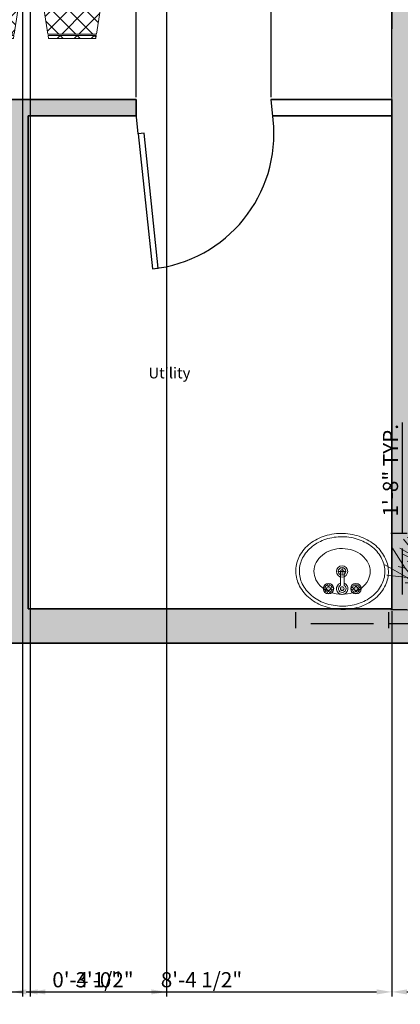
# Model space of a CAD drawing. Units: inches. Extents: x 1872 to 2380, y 714 to 1327.
# Tile 2 of 9: x 2100 to 2200, y 714 to 974. Entities that reach past the tile are written whole.
import ezdxf

# ---------------------------------------------------------------- set-up
doc = ezdxf.new("R2010")
doc.units = ezdxf.units.IN
doc.linetypes.add('HIDDEN', pattern=[9.525, 6.35, -3.175])
for name, color, linetype, lineweight in [('A-ANNO-DIMS', 2, 'Continuous', 18), ('A-AREA-IDEN', 7, 'Continuous', 18), ('A-DOOR', 4, 'Continuous', 25), ('A-FLOR-FIXT', 9, 'Continuous', 20), ('A-FURN', 8, 'Continuous', 18), ('A-WALL', 7, 'Continuous', 35), ('A-WALL-HIDN', 7, 'HIDDEN', 18), ('L-PLNT', 3, 'Continuous', 13)]:
    doc.layers.add(name, color=color, linetype=linetype, lineweight=lineweight)
for name, color, linetype, lineweight, true_color in [('A-FLOR-FIXT-PATT', 7, 'Continuous', 13, 0xd1ffff), ('A-FURN-PATT', 254, 'Continuous', 13, 0xf8ceb3), ('A-WALL-PATT', 242, 'Continuous', 13, 0xd52e31)]:
    doc.layers.add(name, color=color, linetype=linetype, lineweight=lineweight, true_color=true_color)
doc.styles.get("Standard").update_dxf_attribs({"font": 'arial.ttf'})
doc.dimstyles.new('ISO-25', dxfattribs={"dimtxt": 4, "dimasz": 4, "dimexe": 1.25, "dimexo": 0.625, "dimtad": 1, "dimdec": 0, "dimlunit": 3, "dimtxsty": 'Standard', "dimcen": 2.5, "dimadec": 0, "dimazin": 0, "dimtfac": 1, "dimtdec": 0, "dimtmove": 0, "dimatfit": 3, "dimfxl": 1, "dimarcsym": 0})

# ---------------------------------------------------------------- blocks, each defined once
blk = doc.blocks.new('*U5')
at = {"transparency": 33554687}
for p, q in [((0, 0), (0, -6)), ((-40, 0), (-40, -6))]:
    blk.add_line(p, q, dxfattribs=at)
blk.add_lwpolyline([(0, 0), (0, 40), (-1.75, 40), (-1.75, 0)], close=True, dxfattribs=at)
blk.add_arc((0, 0), 40, 90, 180, dxfattribs=at)
blk = doc.blocks.new('Sink - Oval top')
for p, q in [((-1, 0), (1, 0)), ((0, 1), (0, -1))]:
    blk.add_line(p, q)
for points in [[(-12.23, 0.39, 0.117634), (-11.46, -3.36, 0.104469), (-8.88, -6.8, 0.090016), (-5.08, -9.07, 0.08192), (-0.32, -10.02, 0.08192), (4.49, -9.38, 0.090016), (8.42, -7.36, 0.104469), (11.22, -4.09, 0.117634), (12.23, -0.39, 0.117634), (11.46, 3.36, 0.104469), (8.88, 6.8, 0.090016), (5.08, 9.07, 0.08192), (0.32, 10.02, 0.08192), (-4.49, 9.38, 0.090016), (-8.42, 7.36, 0.104469), (-11.22, 4.09, 0.117634)], [(-11.29, 0.16, 0.118622), (-10.52, -3.25, 0.104678), (-8.07, -6.36, 0.089562), (-4.54, -8.37, 0.081185), (-0.13, -9.15, 0.081185), (4.3, -8.49, 0.089562), (7.89, -6.58, 0.104678), (10.42, -3.55, 0.118622), (11.29, -0.16, 0.118622), (10.52, 3.25, 0.104678), (8.07, 6.36, 0.089562), (4.54, 8.37, 0.081185), (0.13, 9.15, 0.081185), (-4.3, 8.49, 0.089562), (-7.89, 6.58, 0.104678), (-10.42, 3.55, 0.118622)], [(-7.42, 0.08, 0.118283), (-6.91, -2.17, 0.104607), (-5.29, -4.21, 0.089718), (-2.97, -5.53, 0.081436), (-0.07, -6.04, 0.081436), (2.84, -5.59, 0.089718), (5.2, -4.33, 0.104607), (6.86, -2.32, 0.118283), (7.42, -0.08, 0.118283), (6.91, 2.17, 0.104607), (5.29, 4.21, 0.089718), (2.97, 5.53, 0.081436), (0.07, 6.04, 0.081436), (-2.84, 5.59, 0.089718), (-5.2, 4.33, 0.104607), (-6.86, 2.32, 0.118283)]]:
    blk.add_lwpolyline(points, format="xyb", close=True)
for radius in [1.5, 1]:
    blk.add_circle((0, 0), radius)
blk = doc.blocks.new('Dining Set - 36 x 72 in.')
for p, q in [((-22, 27.5), (-22.1562, 26.50042)), ((-22, 27.5), (-6, 27.5)), ((-5.8437, 26.49966), (-6, 27.5)), ((6, 27.5), (5.8438, 26.50042)), ((6, 27.5), (22, 27.5)), ((22.1563, 26.49966), (22, 27.5)), ((-22.2343, 26.00059), (-23.4847, 17.99762)), ((-22.2304, 26), (-5.7608, 26)), ((-5.8416, 26.5), (-22.1534, 26.5)), ((-4.5152, 17.99762), (-5.7655, 25.99926)), ((5.7657, 26.00059), (4.5153, 17.99762)), ((5.7696, 26), (22.2392, 26)), ((22.1584, 26.5), (5.8466, 26.5)), ((23.4848, 17.99762), (22.2345, 25.99926)), ((36, 18), (-36, 18)), ((-36, 18), (-36, -18)), ((36, -18), (36, 18)), ((-45.5, 8), (-44.5004, 8.15617)), ((-45.5, 8), (-45.5, -8)), ((-44.5, -8.15843), (-44.5, 8.15338)), ((-44.0006, 8.23428), (-35.9976, 9.48474)), ((-44, 8.23041), (-44, -8.23915)), ((44.0006, 8.23428), (35.9976, 9.48474)), ((44, 8.23041), (44, -8.23915)), ((44.5, -8.15843), (44.5, 8.15338)), ((45.5, 8), (44.5005, 8.15617)), ((45.5, 8), (45.5, -8)), ((-44.4997, -8.15631), (-45.5, -8)), ((-35.9976, -9.48476), (-43.9993, -8.2345)), ((35.9976, -9.48476), (43.9993, -8.2345)), ((44.4997, -8.15631), (45.5, -8)), ((-36, -18), (36, -18)), ((-22.2343, -26.0006), (-23.4847, -17.99762)), ((-4.5152, -17.99762), (-5.7655, -25.99928)), ((5.7657, -26.0006), (4.5153, -17.99762)), ((23.4848, -17.99762), (22.2345, -25.99928)), ((-22.2304, -26), (-5.7608, -26)), ((-22, -27.5), (-22.1562, -26.50044)), ((-5.8416, -26.5), (-22.1534, -26.5)), ((-5.8437, -26.49967), (-6, -27.5)), ((5.7696, -26), (22.2392, -26)), ((6, -27.5), (5.8438, -26.50044)), ((22.1584, -26.5), (5.8466, -26.5)), ((22.1563, -26.49967), (22, -27.5)), ((-22, -27.5), (-6, -27.5)), ((6, -27.5), (22, -27.5))]:
    blk.add_line(p, q)
for points in [[(-36, 15), (-31.1772, 14.97754), (-26.8079, 14.91406), (-22.8538, 14.81543), (-19.276, 14.6875), (-16.0362, 14.53613), (-13.0957, 14.36718), (-10.4159, 14.18652), (-7.9583, 14), (-5.6904, 13.81315), (-3.6035, 13.63021), (-1.6954, 13.45508), (0.0365, 13.29166), (1.5945, 13.14388), (2.9811, 13.01562), (4.1988, 12.9108), (5.25, 12.83333), (6.1393, 12.78613), (6.8802, 12.76823), (7.4883, 12.77767), (7.9792, 12.8125), (8.3685, 12.87077), (8.6719, 12.95052), (8.9049, 13.0498), (9.0833, 13.16666), (9.2205, 13.29899), (9.3216, 13.44401), (9.3895, 13.59879), (9.4271, 13.76041), (9.4373, 13.92594), (9.4232, 14.09245), (9.3875, 14.257), (9.3333, 14.41666), (9.2638, 14.56917), (9.1836, 14.71484), (9.0975, 14.85465), (9.0104, 14.98958), (8.9272, 15.1206), (8.8529, 15.2487), (8.7922, 15.37483), (8.75, 15.5), (8.7305, 15.62467), (8.7344, 15.74739), (8.7617, 15.86621), (8.8125, 15.97916), (8.8867, 16.08431), (8.9844, 16.17968), (9.1055, 16.26334), (9.25, 16.33333), (9.4189, 16.38802), (9.6172, 16.42708), (9.8506, 16.45052), (10.125, 16.45833), (10.4463, 16.45052), (10.8203, 16.42708), (11.2529, 16.38802), (11.75, 16.33333), (12.3184, 16.26318), (12.9694, 16.17838), (13.7151, 16.07991), (14.5677, 15.96875), (15.5395, 15.84586), (16.6426, 15.71224), (17.8893, 15.56884), (19.2917, 15.41666), (20.859, 15.25667), (22.5879, 15.08984), (24.4721, 14.91715), (26.5052, 14.73958), (28.6809, 14.5581), (30.9929, 14.3737), (33.4347, 14.18733), (36, 14)], [(-36, 10), (-28.9766, 10.14274), (-23.1725, 10.20442), (-18.4241, 10.19775), (-14.5677, 10.13541), (-11.4399, 10.03011), (-8.877, 9.89453), (-6.7154, 9.74137), (-4.7917, 9.58333), (-2.9698, 9.43082), (-1.2246, 9.28515), (0.4415, 9.14534), (2.026, 9.01041), (3.5266, 8.87939), (4.9408, 8.7513), (6.266, 8.62516), (7.5, 8.5), (8.6411, 8.37549), (9.6914, 8.2539), (10.6538, 8.13818), (11.5312, 8.03125), (12.3267, 7.93603), (13.043, 7.85547), (13.6831, 7.79248), (14.25, 7.75), (14.7471, 7.7303), (15.1797, 7.73307), (15.5537, 7.75732), (15.875, 7.80208), (16.1494, 7.86637), (16.3828, 7.94922), (16.5811, 8.04964), (16.75, 8.16666), (16.8944, 8.29915), (17.0143, 8.44531), (17.1089, 8.60319), (17.1771, 8.77083), (17.218, 8.94629), (17.2305, 9.1276), (17.2137, 9.31282), (17.1667, 9.5), (17.0895, 9.6875), (16.987, 9.875), (16.8649, 10.0625), (16.7292, 10.25), (16.5856, 10.4375), (16.4401, 10.625), (16.2985, 10.8125), (16.1667, 11), (16.05, 11.18733), (15.9518, 11.3737), (15.8752, 11.5581), (15.8229, 11.73958), (15.798, 11.91715), (15.8034, 12.08984), (15.842, 12.25667), (15.9167, 12.41666), (16.0295, 12.56836), (16.1784, 12.70833), (16.3605, 12.83268), (16.5729, 12.9375), (16.8127, 13.01888), (17.0768, 13.07291), (17.3625, 13.0957), (17.6667, 13.08333), (17.9894, 13.03312), (18.3418, 12.94726), (18.7382, 12.82918), (19.1927, 12.68229), (19.7195, 12.51001), (20.3327, 12.31575), (21.0465, 12.10294), (21.875, 11.875), (22.8357, 11.63354), (23.959, 11.37304), (25.2786, 11.08618), (26.8282, 10.76562), (28.6414, 10.40405), (30.752, 9.99414), (33.1936, 9.52856), (36, 9)], [(-36, 5.5), (-30.7157, 5.3348), (-26.069, 5.20963), (-21.9946, 5.11767), (-18.4271, 5.05208), (-15.3009, 5.00602), (-12.5508, 4.97265), (-10.1112, 4.94515), (-7.9167, 4.91666), (-5.909, 4.88167), (-4.0586, 4.83984), (-2.3429, 4.79215), (-0.7396, 4.73958), (0.7739, 4.6831), (2.22, 4.6237), (3.6213, 4.56233), (5, 4.5), (6.373, 4.43782), (7.7344, 4.3776), (9.0723, 4.32129), (10.375, 4.27083), (11.6309, 4.22819), (12.8281, 4.19531), (13.9551, 4.17415), (15, 4.16666), (15.954, 4.17448), (16.819, 4.19791), (17.6001, 4.23698), (18.3021, 4.29166), (18.9299, 4.36198), (19.4883, 4.44791), (19.9823, 4.54948), (20.4167, 4.66666), (20.7969, 4.79899), (21.1302, 4.94401), (21.4245, 5.09879), (21.6875, 5.26041), (21.9271, 5.42594), (22.1511, 5.59245), (22.3672, 5.757), (22.5834, 5.91666), (22.8065, 6.06868), (23.0404, 6.21093), (23.2879, 6.34147), (23.5521, 6.45833), (23.8358, 6.55957), (24.142, 6.64323), (24.4735, 6.70735), (24.8334, 6.75), (25.2235, 6.76969), (25.642, 6.76692), (26.0858, 6.74267), (26.5521, 6.69791), (27.0379, 6.63362), (27.5404, 6.55078), (28.0565, 6.45036), (28.5834, 6.33333), (29.1242, 6.19987), (29.7071, 6.04687), (30.3661, 5.87044), (31.1354, 5.66666), (32.0493, 5.43164), (33.142, 5.16146), (34.4475, 4.85221), (36, 4.5)], [(-36, -1), (-30.7915, -0.6591), (-26.0195, -0.38216), (-21.6519, -0.16284), (-17.6563, 0.00521), (-14.0005, 0.12833), (-10.6523, 0.21289), (-7.5796, 0.26522), (-4.75, 0.29166), (-2.134, 0.29793), (0.2878, 0.28711), (2.5317, 0.26163), (4.6146, 0.22396), (6.5529, 0.17651), (8.3633, 0.12174), (10.0623, 0.06209), (11.6667, 0), (13.1899, -0.06201), (14.6341, -0.1211), (15.9982, -0.17432), (17.2813, -0.21875), (18.4823, -0.25147), (19.6003, -0.26953), (20.6343, -0.27002), (21.5834, -0.25), (22.4481, -0.20768), (23.2357, -0.14584), (23.9549, -0.06836), (24.6146, 0.02083), (25.2235, 0.11784), (25.7904, 0.21875), (26.3241, 0.31966), (26.8334, 0.41666), (27.3265, 0.50618), (27.8099, 0.58593), (28.2894, 0.65397), (28.7709, 0.70833), (29.2601, 0.74707), (29.763, 0.76823), (30.2855, 0.76985), (30.8334, 0.75), (31.4088, 0.70784), (31.9994, 0.64713), (32.589, 0.57275), (33.1615, 0.48958), (33.7008, 0.4025), (34.1908, 0.3164), (34.6153, 0.23616), (34.9584, 0.16666), (35.2099, 0.11165), (35.3848, 0.07031), (35.504, 0.04069), (35.5886, 0.02083), (35.6594, 0.00879), (35.7377, 0.0026), (35.8442, 0.00032), (36, 0)], [(-36, -6.5), (-27.1843, -6.31267), (-20.084, -6.1263), (-14.469, -5.9419), (-10.1094, -5.76042), (-6.7752, -5.58285), (-4.2363, -5.41016), (-2.2629, -5.24333), (-0.625, -5.08334), (0.8708, -4.93099), (2.2715, -4.78646), (3.5872, -4.64974), (4.8281, -4.52084), (6.0046, -4.39974), (7.127, -4.28646), (8.2053, -4.18099), (9.25, -4.08334), (10.2705, -3.99382), (11.2734, -3.91407), (12.2647, -3.84603), (13.25, -3.79167), (14.2354, -3.75293), (15.2266, -3.73177), (16.2295, -3.73015), (17.25, -3.75), (18.2912, -3.79248), (19.3451, -3.85547), (20.4009, -3.93604), (21.4479, -4.03125), (22.4754, -4.13819), (23.4727, -4.25391), (24.4289, -4.37549), (25.3334, -4.5), (26.1785, -4.62492), (26.9694, -4.74935), (27.7145, -4.87281), (28.4219, -4.99479), (29.1, -5.11483), (29.7572, -5.23242), (30.4016, -5.34709), (31.0417, -5.45834), (31.6837, -5.56437), (32.3262, -5.65821), (32.9658, -5.73153), (33.599, -5.77604), (34.2224, -5.78345), (34.8327, -5.74545), (35.4264, -5.65373), (36, -5.5)], [(-36, -10), (-26.4022, -9.81299), (-18.4675, -9.62891), (-11.9839, -9.45069), (-6.7396, -9.28125), (-2.5226, -9.12354), (0.8789, -8.98047), (3.6769, -8.85498), (6.0833, -8.75), (8.2767, -8.66765), (10.3021, -8.60677), (12.1712, -8.56543), (13.8958, -8.54167), (15.4876, -8.53353), (16.9583, -8.53907), (18.3197, -8.55632), (19.5834, -8.58334), (20.7616, -8.61841), (21.8685, -8.66081), (22.9188, -8.71004), (23.9271, -8.76563), (24.9081, -8.82707), (25.8763, -8.89388), (26.8465, -8.96558), (27.8334, -9.04167), (28.8474, -9.12118), (29.8828, -9.20117), (30.93, -9.27824), (31.9792, -9.34896), (33.0205, -9.40991), (34.0443, -9.45768), (35.0407, -9.48885), (36, -9.5)], [(-36, -14.5), (-30.0881, -14.33513), (-25.0332, -14.21224), (-20.7312, -14.12647), (-17.0781, -14.07292), (-13.97, -14.04671), (-11.3027, -14.04297), (-8.9724, -14.05681), (-6.875, -14.08334), (-4.9224, -14.11833), (-3.0905, -14.16016), (-1.3709, -14.20785), (0.2448, -14.26042), (1.7647, -14.3169), (3.1973, -14.3763), (4.5507, -14.43767), (5.8333, -14.5), (7.0554, -14.5621), (8.235, -14.62175), (9.3922, -14.67652), (10.5469, -14.72396), (11.7192, -14.76164), (12.929, -14.78711), (14.1965, -14.79794), (15.5417, -14.79167), (16.9933, -14.76424), (18.6152, -14.70508), (20.4804, -14.60197), (22.6615, -14.44271), (25.2312, -14.21509), (28.2624, -13.9069), (31.8277, -13.50594), (36, -13)]]:
    blk.add_lwpolyline(points)
blk = doc.blocks.new('Faucet - Bathroom top')
for p, q in [((-4.107, 0.125), (-4.375, 0.125)), ((-3.75, 0.4788), (-3.75, 0.75)), ((-3.5, 0.482), (-3.5, 0.75)), ((-3.1461, 0.125), (-2.875, 0.125)), ((3.143, 0.125), (2.875, 0.125)), ((3.5, 0.4788), (3.5, 0.75)), ((3.75, 0.482), (3.75, 0.75)), ((4.1039, 0.125), (4.375, 0.125)), ((-4.1039, -0.125), (-4.375, -0.125)), ((-3.75, -0.4821), (-3.75, -0.75)), ((-3.5, -0.4789), (-3.5, -0.75)), ((-3.143, -0.125), (-2.875, -0.125)), ((-0.5, -0.8639), (-0.5, -4.5)), ((0.5, -4.5), (0.5, -0.8631)), ((3.1461, -0.125), (2.875, -0.125)), ((3.5, -0.4821), (3.5, -0.75)), ((3.75, -0.4789), (3.75, -0.75)), ((4.107, -0.125), (4.375, -0.125))]:
    blk.add_line(p, q)
for centre, radius in [((-3.625, 0), 1.375), ((-4.625, 0), 0.2795), ((-3.625, 0), 0.5), ((-3.625, 1), 0.2795), ((-2.625, 0), 0.2795), ((0, 0), 0.5), ((3.625, 0), 1.375), ((2.625, 0), 0.2795), ((3.625, 0), 0.5), ((3.625, 1), 0.2795), ((4.625, 0), 0.2795), ((-3.625, -1), 0.2795), ((3.625, -1), 0.2795)]:
    blk.add_circle(centre, radius)
for centre, radius, start, end in [((-3.625, 0), 1, 105.2407, 164.2093), ((-3.625, 0), 1, 16.44125, 74.07887), ((0, 0), 1.5, 289.6514, 250.3603), ((0, 0), 1, 300.3431, 239.7554), ((3.625, 0), 1, 106.12, 164.0884), ((3.625, 0), 1, 16.23422, 73.90469), ((-3.625, 0), 1, 196.2342, 253.9047), ((-3.625, 0), 1, 286.12, 344.0884), ((3.625, 0), 1, 196.4413, 254.0789), ((3.625, 0), 1, 285.2407, 344.2093), ((0, -4.5), 0.5, 180, 0)]:
    blk.add_arc(centre, radius, start, end)
blk = doc.blocks.new('*U18')
for p, q in [((-316.7634, 502.285), (-327.6092, 559.9176)), ((-286.512, 498.3226), (-307.4416, 538.0736)), ((-290.3982, 464.5406), (-265.6078, 577.8246)), ((-207.264, 451.104), (-268.224, 548.64)), ((-240.792, 502.285), (-228.3968, 573.8368)), ((-182.88, 499.872), (-158.496, 536.448)), ((-129.1844, 450.6214), (-140.0302, 542.036)), ((-134.112, 487.68), (-97.536, 548.64)), ((-85.7758, 472.4908), (-73.3552, 548.005)), ((-12.9032, 555.9552), (-2.0574, 522.1732)), ((-5.1562, 486.3846), (2.5908, 542.036)), ((-0.508, 508.254), (22.7584, 536.067)), ((1.0414, 526.1356), (35.1536, 559.9176)), ((2.5908, 542.036), (21.209, 555.9552)), ((-426.72, 414.528), (-475.488, 475.488)), ((-377.952, 463.296), (-451.104, 487.68)), ((-426.72, 414.528), (-390.144, 499.872)), ((-377.952, 463.296), (-329.184, 524.256)), ((-207.264, 304.8), (-377.952, 463.296)), ((-338.455, 424.7896), (-290.3982, 464.5406)), ((-296.5958, 484.4034), (-316.7634, 502.285)), ((-305.8922, 396.9512), (-302.7934, 478.4344)), ((-302.7934, 478.4344), (-270.256, 518.1854)), ((-268.7066, 458.5716), (-250.0884, 500.3038)), ((-182.88, 499.872), (-219.456, 512.064)), ((-207.264, 451.104), (-134.112, 487.68)), ((-121.92, 414.528), (-182.88, 499.872)), ((-73.152, 329.184), (-109.728, 499.872)), ((-97.536, 426.72), (-24.384, 524.256)), ((-70.2564, 426.7708), (-85.7758, 472.4908)), ((-73.152, 402.336), (-60.96, 512.064)), ((8.7884, 335.3562), (-5.1562, 486.3846)), ((-3.6068, 492.3536), (14.986, 518.1854)), ((33.6042, 412.8516), (92.5068, 464.5406)), ((-463.296, 280.416), (-552.577, 423.037)), ((-329.184, 316.992), (-499.872, 414.528)), ((-426.72, 316.992), (-426.72, 414.528)), ((-329.184, 316.992), (-207.264, 451.104)), ((-304.3428, 426.7708), (-268.7066, 458.5716)), ((-182.88, 377.952), (-97.536, 426.72)), ((-85.7758, 389.001), (-129.1844, 452.6026)), ((-24.384, 268.224), (-73.152, 402.336)), ((8.7884, 335.3562), (33.6042, 412.8516)), ((36.576, 390.144), (73.152, 438.912)), ((60.96, 390.144), (85.344, 414.528)), ((-353.568, 316.992), (-487.68, 377.952)), ((-195.072, 316.992), (-182.88, 377.952)), ((-12.192, 274.32), (8.7884, 335.3562)), ((24.384, 304.8), (36.576, 390.144)), ((24.384, 304.8), (73.152, 377.952)), ((48.768, 341.376), (60.96, 390.144)), ((-451.104, 219.456), (-601.0402, 303.8094)), ((-463.296, 280.416), (-512.064, 292.608)), ((-402.336, 207.264), (-463.296, 280.416)), ((-426.72, 316.992), (-451.104, 329.184)), ((-402.336, 207.264), (-426.72, 316.992)), ((-329.184, 316.992), (-353.568, 316.992)), ((-268.224, 109.728), (-329.184, 316.992)), ((-219.456, 195.072), (-207.264, 304.8)), ((-170.688, 219.456), (-195.072, 316.992)), ((-85.344, 134.112), (-73.152, 329.184)), ((-48.768, 243.84), (24.384, 304.8)), ((-451.104, 219.456), (-587.4512, 234.2388)), ((-377.952, 146.304), (-451.104, 219.456)), ((-377.952, 146.304), (-402.336, 207.264)), ((-146.304, 134.112), (-170.688, 219.456)), ((-109.728, 73.152), (-48.768, 243.84)), ((-414.528, 182.88), (-463.296, 182.88)), ((-329.184, 121.92), (-377.952, 146.304)), ((-268.224, 109.728), (-219.456, 195.072)), ((-158.496, 73.152), (-146.304, 134.112)), ((-292.608, 60.96), (-329.184, 121.92)), ((-219.456, 48.768), (-268.224, 109.728)), ((-219.456, 24.384), (-109.728, 73.152)), ((-219.456, 24.384), (-158.496, 73.152)), ((-402.336, 12.192), (-451.104, 0)), ((-341.376, 12.192), (-402.336, 12.192)), ((-243.84, 24.384), (-341.376, 12.192)), ((-243.84, 24.384), (-329.184, 0)), ((-219.456, 24.384), (-292.608, 60.96)), ((-243.84, 24.384), (-195.072, 24.384)), ((-219.456, 24.384), (-219.456, 48.768)), ((-219.456, 24.384), (-73.152, 24.384)), ((-195.072, 24.384), (-158.496, 12.192)), ((-158.496, 12.192), (-85.344, 0)), ((-73.152, 24.384), (0, 0))]:
    blk.add_line(p, q)
blk = doc.blocks.new('*D30')
at = {"layer": 'A-ANNO-DIMS', "color": 0, "lineweight": -2, "transparency": 16777216}
for p, q in [((2172.51, 817.84), (2172.51, 813.54)), ((2197.06, 817.84), (2197.06, 813.54)), ((2176.51, 814.79), (2193.06, 814.79)), ((2197.06, 814.79), (2254.16, 814.79))]:
    blk.add_line(p, q, dxfattribs=at)
at = {"layer": 'A-ANNO-DIMS', "color": 0, "transparency": 16777216}
for points in [[(2176.51, 815.45), (2176.51, 814.12), (2172.51, 814.79)], [(2193.06, 815.45), (2193.06, 814.12), (2197.06, 814.79)]]:
    blk.add_solid(points, dxfattribs=at)
at = {"layer": 'Defpoints', "color": 0, "transparency": 16777216}
for p in [(2172.51, 818.47), (2197.06, 818.47), (2197.06, 814.79)]:
    blk.add_point(p, dxfattribs=at)
at = {"layer": 'A-ANNO-DIMS', "color": 0, "transparency": 16777216, "insert": (2227.61, 817.48), "char_height": 4, "attachment_point": 5}
blk.add_mtext('BASIN 2\'-0 1/2" TYP.', dxfattribs=at)
blk = doc.blocks.new('*D31')
at = {"layer": 'A-ANNO-DIMS', "color": 0, "lineweight": -2, "transparency": 16777216}
for p, q in [((2200.74, 838.61), (2200.74, 867.86)), ((2197.68, 838.61), (2201.99, 838.61)), ((2200.74, 822.47), (2200.74, 834.61)), ((2197.68, 818.47), (2201.99, 818.47))]:
    blk.add_line(p, q, dxfattribs=at)
at = {"layer": 'A-ANNO-DIMS', "color": 0, "transparency": 16777216}
for points in [[(2200.07, 834.61), (2201.41, 834.61), (2200.74, 838.61)], [(2200.07, 822.47), (2201.41, 822.47), (2200.74, 818.47)]]:
    blk.add_solid(points, dxfattribs=at)
at = {"layer": 'Defpoints', "color": 0, "transparency": 16777216}
for p in [(2197.06, 838.61), (2200.74, 838.61), (2197.06, 818.47)]:
    blk.add_point(p, dxfattribs=at)
at = {"layer": 'A-ANNO-DIMS', "color": 0, "transparency": 16777216, "insert": (2198.07, 855.23), "char_height": 4, "attachment_point": 5, "rotation": 90}
blk.add_mtext('1\'-8" TYP.', dxfattribs=at)
blk = doc.blocks.new('*D60')
at = {"layer": 'A-ANNO-DIMS', "color": 0, "lineweight": -2, "transparency": 16777216}
for p, q in [((2097.4, 818.02), (2097.4, 716.39)), ((2197.9, 818.02), (2197.9, 716.39)), ((2101.4, 717.64), (2193.9, 717.64))]:
    blk.add_line(p, q, dxfattribs=at)
at = {"layer": 'A-ANNO-DIMS', "color": 0, "transparency": 16777216}
for points in [[(2101.4, 718.3), (2101.4, 716.97), (2097.4, 717.64)], [(2193.9, 718.3), (2193.9, 716.97), (2197.9, 717.64)]]:
    blk.add_solid(points, dxfattribs=at)
at = {"layer": 'Defpoints', "color": 0, "transparency": 16777216}
for p in [(2097.4, 818.64), (2197.9, 818.64), (2197.9, 717.64)]:
    blk.add_point(p, dxfattribs=at)
at = {"layer": 'A-ANNO-DIMS', "color": 0, "transparency": 16777216, "insert": (2147.65, 720.33), "char_height": 4, "attachment_point": 5}
blk.add_mtext('8\'-4 1/2"', dxfattribs=at)
blk = doc.blocks.new('*D61')
at = {"layer": 'A-ANNO-DIMS', "color": 0, "lineweight": -2, "transparency": 16777216}
for p, q in [((2197.9, 818.02), (2197.9, 716.39)), ((2295.4, 809.02), (2295.4, 716.39)), ((2201.9, 717.64), (2291.4, 717.64))]:
    blk.add_line(p, q, dxfattribs=at)
at = {"layer": 'A-ANNO-DIMS', "color": 0, "transparency": 16777216}
for points in [[(2201.9, 718.3), (2201.9, 716.97), (2197.9, 717.64)], [(2291.4, 718.3), (2291.4, 716.97), (2295.4, 717.64)]]:
    blk.add_solid(points, dxfattribs=at)
at = {"layer": 'Defpoints', "color": 0, "transparency": 16777216}
for p in [(2197.9, 818.64), (2295.4, 809.64), (2295.4, 717.64)]:
    blk.add_point(p, dxfattribs=at)
at = {"layer": 'A-ANNO-DIMS', "color": 0, "transparency": 16777216, "insert": (2246.65, 720.33), "char_height": 4, "attachment_point": 5}
blk.add_mtext('8\'-1 1/2"', dxfattribs=at)
blk = doc.blocks.new('*D70')
at = {"layer": 'A-ANNO-DIMS', "color": 0, "lineweight": -2, "transparency": 16777216}
for p, q in [((2102.4, 1143.52), (2102.4, 716.39)), ((2138.4, 1143.52), (2138.4, 716.39)), ((2106.4, 717.64), (2134.4, 717.64))]:
    blk.add_line(p, q, dxfattribs=at)
at = {"layer": 'A-ANNO-DIMS', "color": 0, "transparency": 16777216}
for points in [[(2106.4, 718.3), (2106.4, 716.97), (2102.4, 717.64)], [(2134.4, 718.3), (2134.4, 716.97), (2138.4, 717.64)]]:
    blk.add_solid(points, dxfattribs=at)
at = {"layer": 'Defpoints', "color": 0, "transparency": 16777216}
for p in [(2102.4, 1144.14), (2138.4, 1144.14), (2138.4, 717.64)]:
    blk.add_point(p, dxfattribs=at)
at = {"layer": 'A-ANNO-DIMS', "color": 0, "transparency": 16777216, "insert": (2120.4, 720.31), "char_height": 4, "attachment_point": 5}
blk.add_mtext('3\'-0"', dxfattribs=at)
blk = doc.blocks.new('*D74')
at = {"layer": 'A-ANNO-DIMS', "color": 0, "lineweight": -2, "transparency": 16777216}
for p, q in [((2130.4, 953.62), (2130.4, 1319.69)), ((2166.01, 953.64), (2166.01, 1319.69)), ((2134.4, 1318.44), (2162.01, 1318.44))]:
    blk.add_line(p, q, dxfattribs=at)
at = {"layer": 'A-ANNO-DIMS', "color": 0, "transparency": 16777216}
for points in [[(2134.4, 1319.11), (2134.4, 1317.78), (2130.4, 1318.44)], [(2162.01, 1319.11), (2162.01, 1317.78), (2166.01, 1318.44)]]:
    blk.add_solid(points, dxfattribs=at)
at = {"layer": 'Defpoints', "color": 0, "transparency": 16777216}
for p in [(2166.01, 1318.44), (2130.4, 952.99), (2166.01, 953.01)]:
    blk.add_point(p, dxfattribs=at)
at = {"layer": 'A-ANNO-DIMS', "color": 0, "transparency": 16777216, "insert": (2148.2, 1321.14), "char_height": 4, "attachment_point": 5}
blk.add_mtext('2\'-11 1/2"', dxfattribs=at)
blk = doc.blocks.new('*D75')
at = {"layer": 'A-ANNO-DIMS', "color": 0, "lineweight": -2, "transparency": 16777216}
for p, q in [((2166.01, 953.64), (2166.02, 983.06)), ((2170.02, 981.81), (2193.91, 981.8)), ((2197.9, 953.62), (2197.91, 983.04))]:
    blk.add_line(p, q, dxfattribs=at)
at = {"layer": 'A-ANNO-DIMS', "color": 0, "transparency": 16777216}
for points in [[(2170.02, 982.48), (2170.02, 981.14), (2166.02, 981.81)], [(2193.91, 982.46), (2193.91, 981.13), (2197.91, 981.79)]]:
    blk.add_solid(points, dxfattribs=at)
at = {"layer": 'Defpoints', "color": 0, "transparency": 16777216}
for p in [(2197.91, 981.79), (2166.01, 953.01), (2197.9, 952.99)]:
    blk.add_point(p, dxfattribs=at)
at = {"layer": 'A-ANNO-DIMS', "color": 0, "transparency": 16777216, "insert": (2181.97, 984.47), "char_height": 4, "attachment_point": 5, "rotation": 359.9714}
blk.add_mtext('2\'-8"', dxfattribs=at)
blk = doc.blocks.new('*D80')
at = {"layer": 'A-ANNO-DIMS', "color": 0, "lineweight": -2, "transparency": 16777216}
for p, q in [((2095.9, 1112.15), (2095.9, 716.39)), ((2100.4, 1112.15), (2100.4, 716.39)), ((2091.9, 717.64), (2087.9, 717.64)), ((2095.9, 717.64), (2100.4, 717.64)), ((2104.4, 717.64), (2129.6, 717.64))]:
    blk.add_line(p, q, dxfattribs=at)
at = {"layer": 'A-ANNO-DIMS', "color": 0, "transparency": 16777216}
for points in [[(2091.9, 718.3), (2091.9, 716.97), (2095.9, 717.64)], [(2104.4, 718.3), (2104.4, 716.97), (2100.4, 717.64)]]:
    blk.add_solid(points, dxfattribs=at)
at = {"layer": 'Defpoints', "color": 0, "transparency": 16777216}
for p in [(2095.9, 1112.77), (2100.4, 1112.77), (2100.4, 717.64)]:
    blk.add_point(p, dxfattribs=at)
at = {"layer": 'A-ANNO-DIMS', "color": 0, "transparency": 16777216, "insert": (2119, 720.33), "char_height": 4, "attachment_point": 5}
blk.add_mtext('0\'-4 1/2"', dxfattribs=at)

msp = doc.modelspace()

# ---------------------------------------------------------------- hatches: boundary and pattern name
at = {"layer": 'A-FLOR-FIXT-PATT', "transparency": 33554687}
h = msp.add_hatch(color=256, dxfattribs=at)
h.dxf.hatch_style = 1
h.paths.add_polyline_path([(2155.91, 1229.14, 0.48008), (2138.39, 1226.79, 0.215004), (2138.39, 1223.5, 0.48008), (2155.91, 1221.14)])
h.paths.add_polyline_path([(2168.91, 1233.64, 0.5), (2167.91, 1234.64), (2163.91, 1234.64, 0.5), (2162.91, 1233.64), (2162.91, 1216.64, 0.5), (2163.91, 1215.64), (2167.91, 1215.64, 0.5), (2168.91, 1216.64)])
h.paths.add_polyline_path([(2285.4, 982.14, 0.5), (2284.4, 983.14), (2267.4, 983.14, 0.5), (2266.4, 982.14), (2266.4, 978.14, 0.5), (2267.4, 977.14), (2284.4, 977.14, 0.5), (2285.4, 978.14)])
h.paths.add_polyline_path([(2277.54, 1007.66, 0.215004), (2274.25, 1007.66, 0.48008), (2271.9, 990.14), (2279.9, 990.14, 0.48008)])
h.paths.add_polyline_path([(2285.9, 985.64), (2282.9, 985.64), (2282.9, 984.14), (2283.9, 984.14), (2283.9, 984.64), (2285.9, 984.64)])
h.paths.add_polyline_path([(2279.53, 1049.02, -0.039819), (2280.2, 1048.28, 0.216904), (2280.37, 1048.66, 0.658258)])
h.paths.add_polyline_path([(2279.53, 1049.02, 0.206085), (2279.37, 1048.66, 0.643515), (2280.2, 1048.28, 0.039819)])
h.paths.add_polyline_path([(2279.37, 1045.03, 1), (2280.37, 1045.03, 1)])
h.paths.add_polyline_path([(2280.37, 1041.41, 0.219955), (2280.19, 1041.79, -0.039801), (2279.52, 1041.05, 0.66578)])
h.paths.add_polyline_path([(2280.19, 1041.79, 0.639405), (2279.37, 1041.41, 0.200639), (2279.52, 1041.05, 0.039801)])
h.paths.add_polyline_path([(2158.34, 1154.61, 1), (2157.34, 1154.61, 1)])
h.paths.add_polyline_path([(2154.72, 1154.61, 1), (2153.72, 1154.61, 1)])
h.paths.add_polyline_path([(2161.97, 1154.61, 1), (2160.97, 1154.61, 1)])
h.paths.add_polyline_path([(2180.69, 824, 1), (2181.69, 824, 1)])
h.paths.add_polyline_path([(2185.32, 824, 1), (2184.32, 824, 1)])
h.paths.add_polyline_path([(2188.94, 824, 1), (2187.94, 824, 1)])
at = {"layer": 'A-FURN-PATT', "transparency": 33554687}
h = msp.add_hatch(dxfattribs=at)
h.set_pattern_fill('ANSI37', color=256)
h.paths.add_polyline_path([(2030.37, 1262.04), (1979.97, 1262.04), (1979.97, 1246.84), (1967.17, 1246.84), (1967.17, 1202.04), (2030.37, 1202.04)])
h.paths.add_polyline_path([(1964.77, 1246.84), (1966.77, 1248.84), (1966.77, 1254.04), (1951.57, 1254.04), (1951.57, 1233.24), (1964.77, 1233.24)])
h.paths.add_polyline_path([(1964.77, 1230.84), (1951.57, 1230.84), (1951.57, 1210.04), (1964.77, 1210.04)])
h.paths.add_polyline_path([(2268.08, 1263.68), (2221.12, 1263.68), (2221.12, 1219.09), (2258.57, 1219.09), (2258.57, 1230.39), (2268.08, 1230.39)])
h.paths.add_polyline_path([(2279.67, 1257.73), (2269.86, 1257.73), (2269.86, 1242.28), (2279.67, 1242.28)])
h.paths.add_polyline_path([(2279.67, 1240.49), (2269.86, 1240.49), (2269.86, 1230.39), (2268.38, 1228.9), (2268.38, 1225.04), (2279.67, 1225.04)])
h.paths.add_polyline_path([(2097.97, 1011.83), (2085.54, 1011.83), (2085.42, 1011.06), (2098.09, 1011.06)])
h.paths.add_polyline_path([(2098.15, 1010.67), (2085.36, 1010.67), (2084.39, 1004.45), (2099.13, 1004.45)])
h.paths.add_polyline_path([(2119.91, 1010.67), (2107.12, 1010.67), (2106.14, 1004.45), (2120.89, 1004.45)])
h.paths.add_polyline_path([(2119.73, 1011.83), (2107.3, 1011.83), (2107.18, 1011.06), (2119.85, 1011.06)])
h.paths.add_polyline_path([(2074.66, 997.83), (2068.44, 996.86), (2068.44, 984.06), (2074.66, 983.09)])
h.paths.add_polyline_path([(2068.05, 996.8), (2067.28, 996.68), (2067.28, 984.25), (2068.05, 984.12)])
h.paths.add_polyline_path([(2136.83, 996.86), (2130.61, 997.83), (2130.61, 983.09), (2136.83, 984.06)])
h.paths.add_polyline_path([(2137.99, 996.68), (2137.22, 996.8), (2137.22, 984.12), (2137.99, 984.25)])
h.paths.add_polyline_path([(2099.13, 976.47), (2084.39, 976.47), (2085.36, 970.26), (2098.15, 970.26)])
h.paths.add_polyline_path([(2120.89, 976.47), (2106.14, 976.47), (2107.12, 970.26), (2119.91, 970.26)])
h.paths.add_polyline_path([(2119.85, 969.87), (2107.18, 969.87), (2107.3, 969.09), (2119.73, 969.09)])
h.paths.add_polyline_path([(2098.09, 969.87), (2085.42, 969.87), (2085.54, 969.09), (2097.97, 969.09)])
at = {"layer": 'A-WALL-PATT', "transparency": 33554687}
h = msp.add_hatch(color=256, dxfattribs=at)
h.dxf.hatch_style = 1
h.paths.add_polyline_path([(2295.4, 1289.64), (1935.4, 1289.64), (1935.4, 809.64), (1949.4, 809.64), (1949.4, 818.64), (1944.4, 818.64), (1944.4, 1108.27), (2100.4, 1108.27), (2100.4, 1112.77), (1944.4, 1112.77), (1944.4, 1280.64), (2095.9, 1280.64), (2095.9, 1141.77), (2100.4, 1141.77), (2100.4, 1280.64), (2169.91, 1280.64), (2169.91, 1244.64), (2169.91, 1160.49, -0.053008), (2170.04, 1158.75, -0.03687), (2169.91, 1157.54), (2169.91, 1148.64), (2167.91, 1148.64), (2138.4, 1148.64), (2138.4, 1144.14), (2167.91, 1144.14), (2174.41, 1144.14), (2174.41, 1280.64), (2197.9, 1280.64), (2197.9, 1184.64), (2202.4, 1184.64), (2202.4, 1280.64), (2286.4, 1280.64), (2286.4, 1148.64), (2197.9, 1148.64), (2197.9, 1108.14), (2202.4, 1108.14), (2202.4, 1144.14), (2286.4, 1144.14), (2286.4, 1060.14), (2202.4, 1060.14), (2202.4, 1108.14), (2197.9, 1108.14), (2197.9, 1060.14), (2197.9, 1053.64), (2202.4, 1053.64), (2202.4, 1055.64), (2286.4, 1055.64), (2286.4, 976.14), (2202.4, 976.14), (2202.4, 1015.64), (2197.9, 1015.64), (2197.9, 971.64), (2197.9, 952.99), (2197.9, 818.64), (2101.9, 818.64), (2101.9, 948.71), (2130.4, 948.71), (2130.4, 952.99), (2073.4, 952.99), (2073.4, 948.71), (2097.4, 948.71), (2097.4, 818.64), (2005.9, 818.64), (2005.9, 948.71), (2029.9, 948.71), (2029.9, 952.99), (2001.4, 952.99), (2001.4, 818.64), (1996.4, 818.64), (1985.23, 818.64), (1985.23, 809.64), (1996.4, 809.64), (2295.4, 809.64)])
h.paths.add_polyline_path([(2202.4, 971.64), (2286.4, 971.64), (2286.4, 858.19), (2286.62, 858.19), (2286.62, 857.19), (2286.4, 857.19), (2286.4, 828.68), (2286.48, 828.76), (2286.4, 828.43), (2286.4, 818.64), (2256.29, 818.64), (2255.29, 818.39), (2254.54, 818.64), (2238.99, 818.64), (2238.75, 818.58), (2238.56, 818.64), (2202.4, 818.64), (2202.4, 952.99)], flags=16)
h.paths.add_polyline_path([(2260.41, 970, -0.15), (2280.41, 970), (2278.41, 967, 0.001913), (2277.92, 967.06), (2277.41, 964.5), (2278.64, 964.5), (2278.72, 964), (2279.41, 964), (2282.41, 953, -0.541163), (2280.76, 950.93), (2280.91, 950, -0.414214), (2279.91, 949), (2279.41, 949), (2279.91, 945), (2278.41, 945), (2277.91, 949), (2270.41, 949), (2262.91, 949), (2262.41, 945), (2260.91, 945), (2261.41, 949), (2260.91, 949, -0.414214), (2259.91, 950), (2260.05, 950.93, -0.505809), (2258.36, 952.83), (2261.41, 964), (2262.1, 964), (2262.17, 964.5), (2263.41, 964.5), (2262.9, 967.06, 0.001913), (2262.41, 967)], flags=0)
h.paths.add_polyline_path([(2257.85, 934.42), (2280.51, 934.42, -0.333333), (2281.77, 933.16), (2281.77, 923.09, -0.333333), (2280.51, 921.83), (2277.57, 921.83), (2277.57, 921.41), (2275.89, 921.41), (2275.89, 921.83), (2262.46, 921.83), (2262.46, 921.41), (2260.79, 921.41), (2260.79, 921.83), (2257.85, 921.83, -0.333333), (2256.59, 923.09), (2256.59, 933.16, -0.333333)], flags=0)
h.paths.add_polyline_path([(2260.61, 912.79), (2262.11, 912.79), (2262.61, 908.79), (2270.11, 908.79), (2277.61, 908.79), (2278.11, 912.79), (2279.61, 912.79), (2279.11, 908.79), (2279.61, 908.79, -0.414214), (2280.61, 907.79), (2280.46, 906.86, -0.505809), (2282.15, 904.96), (2279.11, 893.79), (2278.42, 893.79), (2278.34, 893.29), (2277.11, 893.29), (2277.62, 890.73, 0.001913), (2278.11, 890.79), (2280.11, 887.79, -0.15), (2260.11, 887.79), (2262.11, 890.79, 0.001913), (2262.59, 890.73), (2263.11, 893.29), (2261.87, 893.29), (2261.79, 893.79), (2261.11, 893.79), (2258.11, 904.79, -0.541163), (2259.75, 906.86), (2259.61, 907.79, -0.414214), (2260.61, 908.79), (2261.11, 908.79)], flags=0)
h.paths.add_polyline_path([(2252.62, 864.69), (2253.62, 864.69), (2253.62, 862.19), (2253.62, 860.69), (2256.62, 859.69, -0.362186), (2259.62, 862.19, -0.174416), (2262.62, 860.69, 0.103487), (2265.62, 859.19, -0.219276), (2266.55, 858.19), (2268.62, 858.19), (2268.62, 859.69), (2267.62, 859.69), (2267.62, 863.69), (2270.12, 863.69), (2270.12, 859.69), (2269.12, 859.69), (2269.12, 858.19), (2274.62, 858.19), (2278.62, 858.19), (2278.62, 862.69), (2275.62, 864.69), (2275.62, 865.69), (2279.62, 862.69), (2279.62, 858.19), (2279.62, 852.69), (2275.62, 849.19), (2275.62, 850.19), (2278.62, 852.69), (2278.62, 857.19), (2274.62, 857.19), (2271.12, 857.19), (2271.12, 855.69), (2272.12, 855.69), (2272.12, 851.69), (2269.62, 851.69), (2269.62, 855.69), (2270.62, 855.69), (2270.62, 857.19), (2266.55, 857.19, -0.219162), (2265.62, 856.19, 0.103506), (2262.62, 854.69, -0.174459), (2259.62, 853.19, -0.362114), (2256.62, 855.69), (2253.62, 854.69), (2253.62, 850.69), (2252.62, 850.69)], flags=0)
h.paths.add_polyline_path([(2253.62, 859.69), (2256.62, 858.69), (2256.62, 856.69), (2253.62, 855.69)], flags=0)
h.paths.add_polyline_path([(2208.62, 838.17), (2208.28, 836.61), (2207.75, 836.18), (2207.67, 833.93), (2208.71, 832.96), (2211.55, 836.09), (2214.43, 837.53), (2214.45, 837.55), (2214.61, 836.16), (2215.48, 834.9), (2215.87, 835.13), (2217.12, 836.79), (2216.83, 834.17), (2218.8, 828.76), (2219.23, 829.13), (2220.06, 831.53), (2219.5, 837.61), (2219.53, 837.66), (2219.68, 838.72), (2219.62, 838.91), (2219.72, 839.01), (2219.51, 837.47), (2219.77, 834.68), (2220.87, 834.05), (2221.03, 834.58), (2222.05, 835.47), (2222.71, 834.65), (2223.67, 836.89), (2224.63, 836.57), (2226.23, 835.08), (2227.55, 836.18), (2227.59, 837.16), (2228.42, 838.17), (2228.08, 836.61), (2227.55, 836.18), (2227.47, 833.93), (2228.51, 832.96), (2231.35, 836.09), (2234.23, 837.53), (2234.25, 837.55), (2234.42, 836.16), (2235.28, 834.9), (2235.67, 835.13), (2236.93, 836.79), (2236.93, 836.84), (2238.69, 834.65), (2239.41, 836.34), (2239.3, 837.61), (2239.34, 837.66), (2239.48, 838.72), (2239.42, 838.91), (2239.52, 839.01), (2239.31, 837.47), (2239.36, 836.98), (2240.61, 836.57), (2242.2, 835.08), (2243.53, 836.18), (2243.57, 837.16), (2244.39, 838.17), (2244.05, 836.61), (2243.53, 836.18), (2243.44, 833.93), (2244.49, 832.96), (2247.33, 836.09), (2250.21, 837.53), (2250.22, 837.55), (2250.39, 836.16), (2251.25, 834.9), (2251.65, 835.13), (2252.9, 836.79), (2252.61, 834.17), (2254.09, 830.08), (2254.54, 829.37), (2254.85, 828.99), (2255.01, 829.13), (2255.83, 831.53), (2255.29, 837.44), (2255.28, 837.44), (2255.46, 838.72), (2255.4, 838.91), (2255.5, 839.01), (2255.28, 837.47), (2255.29, 837.44), (2257.9, 836.57), (2259.5, 835.08), (2260.82, 836.18), (2260.86, 837.16), (2261.69, 838.17), (2261.35, 836.61), (2260.82, 836.18), (2260.74, 833.93), (2261.78, 832.96), (2264.62, 836.09), (2267.5, 837.53), (2267.52, 837.55), (2267.68, 836.16), (2268.54, 834.9), (2268.94, 835.13), (2270.19, 836.79), (2269.9, 834.17), (2271.79, 828.96), (2271.98, 828.86), (2272.3, 829.13), (2273.13, 831.53), (2272.56, 837.61), (2272.6, 837.66), (2272.75, 838.72), (2272.69, 838.91), (2272.79, 839.01), (2272.58, 837.47), (2273.13, 831.53), (2273.02, 831.22), (2273.67, 831.01), (2273.92, 831.6), (2273.83, 830.95), (2274.1, 830.86), (2275.75, 833.35), (2276.03, 831.86), (2276.57, 831.38), (2277, 831.91), (2277.3, 833.27), (2279.06, 830.44), (2281.09, 831.46), (2281.1, 831.48), (2281.21, 830.5), (2281.82, 829.61), (2282.1, 829.77), (2282.98, 830.94), (2282.77, 829.1), (2284.15, 825.3), (2284.46, 825.55), (2285.04, 827.24), (2284.64, 831.51), (2284.67, 831.55), (2284.77, 832.3), (2284.73, 832.43), (2284.8, 832.5), (2284.65, 831.42), (2285.04, 827.24), (2284.46, 825.55), (2283.45, 824.71), (2281.76, 819.99), (2278.73, 818.64), (2276.7, 819.65), (2275.69, 821.34), (2274.34, 822.01), (2272.32, 824.04), (2269.58, 824.33), (2268.46, 821.21), (2264.14, 819.29), (2261.26, 820.73), (2259.82, 823.13), (2257.9, 824.09), (2255.02, 826.97), (2253.29, 827.15), (2251.17, 821.21), (2246.85, 819.29), (2243.97, 820.73), (2242.53, 823.13), (2240.61, 824.09), (2237.73, 826.97), (2237.27, 827.01), (2235.19, 821.21), (2230.87, 819.29), (2227.99, 820.73), (2226.55, 823.13), (2224.63, 824.09), (2221.75, 826.97), (2217.61, 827.41), (2215.39, 821.21), (2211.07, 819.29), (2208.19, 820.73), (2206.75, 823.13), (2204.83, 824.09), (2203.87, 826.49), (2202.91, 830.81), (2202.91, 834.65), (2203.87, 836.89), (2204.83, 836.57), (2206.43, 835.08), (2207.75, 836.18), (2207.79, 837.16)], flags=0)
h.paths.add_polyline_path([(2221.04, 832.88), (2221.82, 832.52), (2222.11, 833.69), (2222.71, 834.29), (2222.71, 832.11), (2225.59, 830.81), (2226.55, 830.81), (2228.95, 822.65), (2230.87, 820.25), (2230.87, 819.29), (2233.27, 821.21), (2233.75, 823.61), (2232.79, 826.97), (2231.99, 830.19), (2236.41, 827.71), (2236.63, 831.29), (2235.93, 834.58), (2242.53, 830.81), (2241.57, 830.81), (2240.97, 831.07), (2240.47, 830.33), (2239.06, 829.14), (2239.65, 826.49), (2237.25, 829.37), (2236.52, 829.55), (2236.41, 827.71), (2231.99, 830.19), (2232.79, 826.97), (2233.75, 823.61), (2233.27, 821.21), (2230.87, 819.29), (2230.87, 820.25), (2228.95, 822.65), (2226.55, 830.81), (2225.59, 830.81), (2222.71, 832.11), (2222.71, 830.81), (2223.67, 826.49), (2221.27, 829.37), (2220.67, 830.33), (2220.67, 830.33)], flags=0)
h.paths.add_polyline_path([(2255.98, 833), (2259.82, 830.81), (2258.86, 830.81), (2257.25, 831.54), (2256.45, 830.33), (2256.66, 831.81), (2256.02, 832.1), (2255.98, 831.99)], flags=0)
h.paths.add_polyline_path([(2275.69, 826.73), (2277.07, 828.25), (2275.46, 829.74), (2276.39, 830.51), (2276.33, 828.93), (2279.06, 826.4), (2278.73, 823.36), (2277.38, 821)], flags=0)
h.paths.add_polyline_path([(2260.6, 925.25), (2276.34, 925.25), (2276.34, 931.01), (2260.6, 931.01)], flags=8)
h.paths.add_polyline_path([(2202.72, 1070.05), (2202.72, 1092.72), (2197.34, 1092.72), (2197.34, 1070.05)], flags=25)

# ---------------------------------------------------------------- linework, layer by layer
at = {"layer": 'A-WALL', "transparency": 33554687}
for p, q in [((2197.9, 1017.64), (2197.9, 971.64)), ((2130.4, 952.99), (2073.4, 952.99)), ((2130.4, 952.99), (2130.4, 948.71)), ((2166.01, 952.99), (2166, 952.99)), ((2197.9, 952.99), (2197.9, 818.64)), ((2101.9, 948.71), (2130.4, 948.71)), ((2166.46, 948.71), (2166.4, 948.71)), ((2166.46, 948.71), (2197.9, 948.71)), ((2197.9, 818.64), (2101.9, 818.64))]:
    msp.add_line(p, q, dxfattribs=at)
at = {"layer": 'A-WALL'}
for p, q in [((2197.9, 952.99), (2166.01, 952.99)), ((2101.9, 948.71), (2101.9, 818.64))]:
    msp.add_line(p, q, dxfattribs=at)
at = {"layer": 'A-WALL', "transparency": 33554687}
msp.add_lwpolyline([(1949.4, 809.64), (1935.4, 809.64), (1935.4, 1289.64), (2295.4, 1289.64), (2295.4, 809.64), (1996.4, 809.64)], dxfattribs=at)
at = {"layer": 'A-WALL-HIDN', "transparency": 33554687}
msp.add_line((2197.9, 952.99), (2197.9, 971.64), dxfattribs=at)

# ---------------------------------------------------------------- block references
at = {"layer": 'A-DOOR', "transparency": 33554687, "xscale": 0.8951335839366908, "yscale": 0.8951335839366908, "zscale": 0.8951335839366908, "rotation": 185.9695437352451}
msp.add_blockref('*U5', (2130.96, 943.95), dxfattribs=at)
at = {"layer": 'A-FLOR-FIXT', "transparency": 33554687}
msp.add_blockref('Sink - Oval top', (2184.78, 828.54), dxfattribs=at)
at = {"layer": 'A-FLOR-FIXT', "transparency": 33554687, "rotation": 180}
msp.add_blockref('Faucet - Bathroom top', (2184.82, 824), dxfattribs=at)
at = {"layer": 'A-FURN', "transparency": 33554687, "xscale": 0.7771303306467578, "yscale": 0.7771303306467578, "zscale": 0.7771303306467578}
msp.add_blockref('Dining Set - 36 x 72 in.', (2102.64, 990.46), dxfattribs=at)
at = {"layer": 'L-PLNT', "transparency": 33554687, "xscale": 0.0393700787401575, "yscale": 0.0393700787401575, "zscale": 0.0393700787401575}
msp.add_blockref('*U18', (2219.71, 818.33), dxfattribs=at)

# ---------------------------------------------------------------- texts
at = {"layer": 'A-AREA-IDEN', "transparency": 33554687}
msp.add_text('Utility', height=2.866, dxfattribs=at).set_placement((2133.65, 879.46))

# ---------------------------------------------------------------- dimensions: what is measured, and where the dimension line sits
at = {"layer": 'A-ANNO-DIMS', "transparency": 33554687}
for base, p1, p2, picture, middle in [((2166.01, 1318.44), (2130.4, 952.99), (2166.01, 953.01), '*D74', (2148.2, 1321.14)), ((2138.4, 717.64), (2102.4, 1144.14), (2138.4, 1144.14), '*D70', (2120.4, 720.31)), ((2100.4, 717.64), (2095.9, 1112.77), (2100.4, 1112.77), '*D80', (2119, 720.33)), ((2197.9, 717.64), (2097.4, 818.64), (2197.9, 818.64), '*D60', (2147.65, 720.33)), ((2295.4, 717.64), (2197.9, 818.64), (2295.4, 809.64), '*D61', (2246.65, 720.33))]:
    dim = msp.add_linear_dim(base=base, p1=p1, p2=p2, dimstyle='ISO-25', override={"dimdec": 1, "dimlfac": 1, "dimrnd": 0, "dimzin": 1, "dimdsep": 46, "dimlunit": 4, "dimfrac": 2}, dxfattribs=at)
    dim.commit()
    dim.dimension.update_dxf_attribs({"geometry": picture, "text_midpoint": middle})
dim = msp.add_linear_dim(base=(2197.91, 981.79), p1=(2166.01, 953.01), p2=(2197.9, 952.99), angle=359.9714, dimstyle='ISO-25', override={"dimdec": 1, "dimlfac": 1, "dimrnd": 0, "dimzin": 1, "dimdsep": 46, "dimlunit": 4, "dimfrac": 2}, dxfattribs=at)
dim.commit()
dim.dimension.update_dxf_attribs({"geometry": '*D75', "text_midpoint": (2181.97, 984.47)})
dim = msp.add_linear_dim(base=(2200.74, 838.61), p1=(2197.06, 818.47), p2=(2197.06, 838.61), angle=90, text='<> TYP.', dimstyle='ISO-25', override={"dimdec": 1, "dimlfac": 1, "dimrnd": 0, "dimzin": 1, "dimdsep": 46, "dimlunit": 4, "dimfrac": 2}, dxfattribs=at)
dim.commit()
dim.dimension.update_dxf_attribs({"geometry": '*D31', "text_midpoint": (2198.07, 855.23)})
dim = msp.add_linear_dim(base=(2197.0578, 814.7862), p1=(2172.5069, 818.4689), p2=(2197.0578, 818.4689), text='BASIN <> TYP.', dimstyle='ISO-25', override={"dimdec": 1, "dimlfac": 1, "dimrnd": 0, "dimzin": 1, "dimdsep": 46, "dimlunit": 4, "dimfrac": 2}, dxfattribs=at)
dim.commit()
dim.dimension.update_dxf_attribs({"geometry": '*D30', "text_midpoint": (2227.6064, 817.4794)})

doc.saveas('drawing.dxf')
